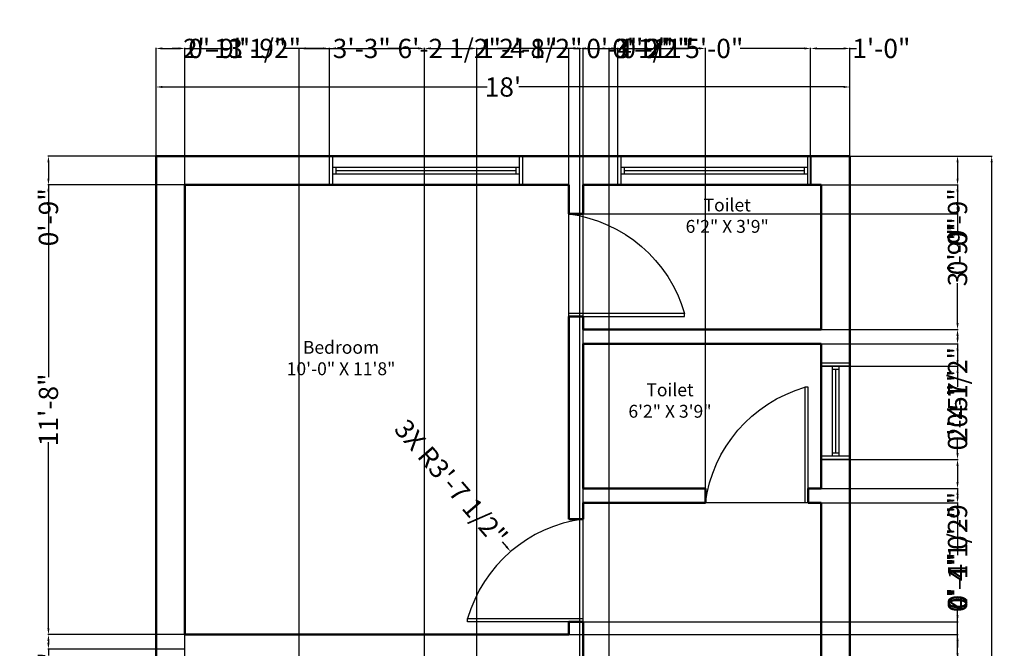
# Model space of a CAD drawing. Units: inches. Extents: x -34 to 296, y -84 to 618.
# Tile 3 of 3: x -11 to 296, y 423 to 618. Entities that reach past the tile are written whole.
import ezdxf

# ---------------------------------------------------------------- set-up
doc = ezdxf.new("R2010")
doc.units = ezdxf.units.IN
doc.header["$LTSCALE"] = 4
doc.header["$MEASUREMENT"] = 0
for name, color, linetype, lineweight in [('A-ANNO-DIMS', 2, 'Continuous', 18), ('A-AREA-IDEN', 3, 'Continuous', 18), ('A-DOOR', 4, 'Continuous', 25), ('A-GLAZ', 3, 'Continuous', 25), ('A-WALL', 7, 'Continuous', 50)]:
    doc.layers.add(name, color=color, linetype=linetype, lineweight=lineweight)
doc.styles.get("Standard").update_dxf_attribs({"font": 'arial.ttf'})
doc.dimstyles.get("Standard").update_dxf_attribs({"dimtxt": 6, "dimasz": 2, "dimexe": 0.18, "dimexo": 0.0625, "dimgap": 0.09, "dimtad": 0, "dimdec": 0, "dimzin": 0, "dimdsep": 46, "dimlunit": 4, "dimtxsty": 'Standard', "dimcen": 0.09, "dimadec": 0, "dimazin": 0, "dimtfac": 1, "dimtdec": 0, "dimtofl": 0, "dimtmove": 0, "dimatfit": 3, "dimfxl": 1, "dimtolj": 1, "dimtzin": 0, "dimarcsym": 0})

# ---------------------------------------------------------------- blocks, each defined once
blk = doc.blocks.new('*D1')
at = {"layer": 'A-ANNO-DIMS', "color": 0, "lineweight": -2, "transparency": 16777216}
for p, q in [((31.47, 576.1), (31.47, 597.71)), ((247.47, 576.1), (247.47, 597.71)), ((33.47, 597.53), (134.57, 597.53)), ((245.47, 597.53), (144.37, 597.53))]:
    blk.add_line(p, q, dxfattribs=at)
at = {"layer": 'A-ANNO-DIMS', "color": 0, "transparency": 16777216}
for points in [[(33.47, 597.86), (33.47, 597.2), (31.47, 597.53)], [(245.47, 597.86), (245.47, 597.2), (247.47, 597.53)]]:
    blk.add_solid(points, dxfattribs=at)
at = {"layer": 'Defpoints', "color": 0, "transparency": 16777216}
for p in [(247.47, 597.53), (31.47, 576.03), (247.47, 576.03)]:
    blk.add_point(p, dxfattribs=at)
at = {"layer": 'A-ANNO-DIMS', "color": 0, "transparency": 16777216, "insert": (139.47, 597.53), "char_height": 6, "attachment_point": 5}
blk.add_mtext("\\A1;18'", dxfattribs=at)
blk = doc.blocks.new('*D2')
at = {"layer": 'A-ANNO-DIMS', "color": 0, "lineweight": -2, "transparency": 16777216}
for p, q in [((247.53, 576.03), (291.77, 576.03)), ((291.59, 574.03), (291.59, 311.33)), ((291.59, 38.03), (291.59, 300.73)), ((247.53, 36.03), (291.77, 36.03))]:
    blk.add_line(p, q, dxfattribs=at)
at = {"layer": 'A-ANNO-DIMS', "color": 0, "transparency": 16777216}
for points in [[(291.26, 574.03), (291.92, 574.03), (291.59, 576.03)], [(291.26, 38.03), (291.92, 38.03), (291.59, 36.03)]]:
    blk.add_solid(points, dxfattribs=at)
at = {"layer": 'Defpoints', "color": 0, "transparency": 16777216}
for p in [(247.47, 576.03), (247.47, 36.03), (291.59, 36.03)]:
    blk.add_point(p, dxfattribs=at)
at = {"layer": 'A-ANNO-DIMS', "color": 0, "transparency": 16777216, "insert": (291.59, 306.03), "char_height": 6, "attachment_point": 5, "rotation": 90}
blk.add_mtext("\\A1;45'", dxfattribs=at)
blk = doc.blocks.new('DOOR')
for p, q in [((177.71, 683.29), (177.71, 692.29)), ((177.71, 692.29), (237.71, 692.29)), ((178.71, 683.29), (178.71, 692.29)), ((236.71, 692.29), (236.71, 683.29)), ((237.71, 692.29), (237.71, 683.29)), ((178.71, 688.79), (236.71, 688.79)), ((178.71, 686.79), (236.71, 686.79)), ((179.71, 686.79), (179.71, 688.79)), ((179.71, 687.79), (235.71, 687.79)), ((235.71, 688.79), (235.71, 686.79)), ((237.71, 683.29), (177.71, 683.29))]:
    blk.add_line(p, q)
blk = doc.blocks.new('DOOR-900')
for p, q in [((36, 0), (36, 32)), ((0, 0), (0, 1)), ((0, 1), (36, 1)), ((36, 0), (0, 0))]:
    blk.add_line(p, q)
blk.add_arc((41.68, -11), 43.37, 97.5204, 163.9438)
blk = doc.blocks.new('*D14')
at = {"layer": 'A-ANNO-DIMS', "color": 0, "lineweight": -2, "transparency": 16777216}
for p, q in [((31.47, 576.1), (31.47, 609.71)), ((33.47, 609.53), (38.47, 609.53)), ((40.47, 567.1), (40.47, 609.71)), ((40.47, 609.53), (42.47, 609.53))]:
    blk.add_line(p, q, dxfattribs=at)
at = {"layer": 'A-ANNO-DIMS', "color": 0, "transparency": 16777216}
for points in [[(33.47, 609.87), (33.47, 609.2), (31.47, 609.53)], [(38.47, 609.87), (38.47, 609.2), (40.47, 609.53)]]:
    blk.add_solid(points, dxfattribs=at)
at = {"layer": 'Defpoints', "color": 0, "transparency": 16777216}
for p in [(40.47, 609.53), (31.47, 576.03), (40.47, 567.03)]:
    blk.add_point(p, dxfattribs=at)
at = {"layer": 'A-ANNO-DIMS', "color": 0, "transparency": 16777216, "insert": (50.53, 609.53), "char_height": 6, "attachment_point": 5}
blk.add_mtext('\\A1;0\'-9"', dxfattribs=at)
blk = doc.blocks.new('*D15')
at = {"layer": 'A-ANNO-DIMS', "color": 0, "lineweight": -2, "transparency": 16777216}
for p, q in [((40.47, 567.1), (40.47, 609.71)), ((42.47, 609.53), (54.92, 609.53)), ((83.5, 609.53), (71.05, 609.53)), ((85.5, 567.1), (85.5, 609.71))]:
    blk.add_line(p, q, dxfattribs=at)
at = {"layer": 'A-ANNO-DIMS', "color": 0, "transparency": 16777216}
for points in [[(42.47, 609.87), (42.47, 609.2), (40.47, 609.53)], [(83.5, 609.87), (83.5, 609.2), (85.5, 609.53)]]:
    blk.add_solid(points, dxfattribs=at)
at = {"layer": 'Defpoints', "color": 0, "transparency": 16777216}
for p in [(85.5, 609.53), (40.47, 567.03), (85.5, 567.03)]:
    blk.add_point(p, dxfattribs=at)
at = {"layer": 'A-ANNO-DIMS', "color": 0, "transparency": 16777216, "insert": (62.99, 609.53), "char_height": 6, "attachment_point": 5}
blk.add_mtext('\\A1;3\'-9"', dxfattribs=at)
blk = doc.blocks.new('*D16')
at = {"layer": 'A-ANNO-DIMS', "color": 0, "lineweight": -2, "transparency": 16777216}
for p, q in [((85.5, 567.1), (85.5, 609.71)), ((87.5, 609.53), (107.66, 609.53)), ((157.97, 609.53), (137.81, 609.53)), ((159.97, 567.1), (159.97, 609.71))]:
    blk.add_line(p, q, dxfattribs=at)
at = {"layer": 'A-ANNO-DIMS', "color": 0, "transparency": 16777216}
for points in [[(87.5, 609.87), (87.5, 609.2), (85.5, 609.53)], [(157.97, 609.87), (157.97, 609.2), (159.97, 609.53)]]:
    blk.add_solid(points, dxfattribs=at)
at = {"layer": 'Defpoints', "color": 0, "transparency": 16777216}
for p in [(159.97, 609.53), (85.5, 567.03), (159.97, 567.03)]:
    blk.add_point(p, dxfattribs=at)
at = {"layer": 'A-ANNO-DIMS', "color": 0, "transparency": 16777216, "insert": (122.74, 609.53), "char_height": 6, "attachment_point": 5}
blk.add_mtext('\\A1;6\'-2 1/2"', dxfattribs=at)
blk = doc.blocks.new('*D17')
at = {"layer": 'A-ANNO-DIMS', "color": 0, "lineweight": -2, "transparency": 16777216}
for p, q in [((159.97, 567.1), (159.97, 609.71)), ((161.97, 609.53), (162.47, 609.53)), ((164.47, 567.1), (164.47, 609.71)), ((164.47, 609.53), (166.47, 609.53))]:
    blk.add_line(p, q, dxfattribs=at)
at = {"layer": 'A-ANNO-DIMS', "color": 0, "transparency": 16777216}
for points in [[(161.97, 609.87), (161.97, 609.2), (159.97, 609.53)], [(162.47, 609.87), (162.47, 609.2), (164.47, 609.53)]]:
    blk.add_solid(points, dxfattribs=at)
at = {"layer": 'Defpoints', "color": 0, "transparency": 16777216}
for p in [(164.47, 609.53), (159.97, 567.03), (164.47, 567.03)]:
    blk.add_point(p, dxfattribs=at)
at = {"layer": 'A-ANNO-DIMS', "color": 0, "transparency": 16777216, "insert": (181.52, 609.53), "char_height": 6, "attachment_point": 5}
blk.add_mtext('\\A1;0\'-4 1/2"', dxfattribs=at)
blk = doc.blocks.new('*D18')
at = {"layer": 'A-ANNO-DIMS', "color": 0, "lineweight": -2, "transparency": 16777216}
for p, q in [((164.47, 567.1), (164.47, 609.71)), ((166.47, 609.53), (173.24, 609.53)), ((175.24, 567.1), (175.24, 609.71)), ((175.24, 609.53), (177.24, 609.53))]:
    blk.add_line(p, q, dxfattribs=at)
at = {"layer": 'A-ANNO-DIMS', "color": 0, "transparency": 16777216}
for points in [[(166.47, 609.87), (166.47, 609.2), (164.47, 609.53)], [(173.24, 609.87), (173.24, 609.2), (175.24, 609.53)]]:
    blk.add_solid(points, dxfattribs=at)
at = {"layer": 'Defpoints', "color": 0, "transparency": 16777216}
for p in [(175.24, 609.53), (164.47, 567.03), (175.24, 567.03)]:
    blk.add_point(p, dxfattribs=at)
at = {"layer": 'A-ANNO-DIMS', "color": 0, "transparency": 16777216, "insert": (187.64, 609.53), "char_height": 6, "attachment_point": 5}
blk.add_mtext('\\A1;0\'-11"', dxfattribs=at)
blk = doc.blocks.new('*D19')
at = {"layer": 'A-ANNO-DIMS', "color": 0, "lineweight": -2, "transparency": 16777216}
for p, q in [((175.24, 567.1), (175.24, 609.71)), ((177.24, 609.53), (197.18, 609.53)), ((233.24, 609.53), (213.31, 609.53)), ((235.24, 567.1), (235.24, 609.71))]:
    blk.add_line(p, q, dxfattribs=at)
at = {"layer": 'A-ANNO-DIMS', "color": 0, "transparency": 16777216}
for points in [[(177.24, 609.87), (177.24, 609.2), (175.24, 609.53)], [(233.24, 609.87), (233.24, 609.2), (235.24, 609.53)]]:
    blk.add_solid(points, dxfattribs=at)
at = {"layer": 'Defpoints', "color": 0, "transparency": 16777216}
for p in [(235.24, 609.53), (175.24, 567.03), (235.24, 567.03)]:
    blk.add_point(p, dxfattribs=at)
at = {"layer": 'A-ANNO-DIMS', "color": 0, "transparency": 16777216, "insert": (205.24, 609.53), "char_height": 6, "attachment_point": 5}
blk.add_mtext('\\A1;5\'-0"', dxfattribs=at)
blk = doc.blocks.new('*D20')
at = {"layer": 'A-ANNO-DIMS', "color": 0, "lineweight": -2, "transparency": 16777216}
for p, q in [((235.24, 567.1), (235.24, 609.71)), ((237.24, 609.53), (245.47, 609.53)), ((247.47, 576.1), (247.47, 609.71)), ((247.47, 609.53), (249.47, 609.53))]:
    blk.add_line(p, q, dxfattribs=at)
at = {"layer": 'A-ANNO-DIMS', "color": 0, "transparency": 16777216}
for points in [[(237.24, 609.87), (237.24, 609.2), (235.24, 609.53)], [(245.47, 609.87), (245.47, 609.2), (247.47, 609.53)]]:
    blk.add_solid(points, dxfattribs=at)
at = {"layer": 'Defpoints', "color": 0, "transparency": 16777216}
for p in [(247.47, 609.53), (247.47, 576.03), (235.24, 567.03)]:
    blk.add_point(p, dxfattribs=at)
at = {"layer": 'A-ANNO-DIMS', "color": 0, "transparency": 16777216, "insert": (257.25, 609.53), "char_height": 6, "attachment_point": 5}
blk.add_mtext('\\A1;1\'-0"', dxfattribs=at)
blk = doc.blocks.new('*D21')
at = {"layer": 'A-ANNO-DIMS', "color": 0, "lineweight": -2, "transparency": 16777216}
for p, q in [((31.4, 576.03), (-2.21, 576.03)), ((-2.03, 574.03), (-2.03, 569.03)), ((40.4, 567.03), (-2.21, 567.03)), ((-2.03, 567.03), (-2.03, 565.03))]:
    blk.add_line(p, q, dxfattribs=at)
at = {"layer": 'A-ANNO-DIMS', "color": 0, "transparency": 16777216}
for points in [[(-2.37, 574.03), (-1.7, 574.03), (-2.03, 576.03)], [(-2.37, 569.03), (-1.7, 569.03), (-2.03, 567.03)]]:
    blk.add_solid(points, dxfattribs=at)
at = {"layer": 'Defpoints', "color": 0, "transparency": 16777216}
for p in [(31.47, 576.03), (-2.03, 567.03), (40.47, 567.03)]:
    blk.add_point(p, dxfattribs=at)
at = {"layer": 'A-ANNO-DIMS', "color": 0, "transparency": 16777216, "insert": (-2.03, 556.97), "char_height": 6, "attachment_point": 5, "rotation": 90}
blk.add_mtext('\\A1;0\'-9"', dxfattribs=at)
blk = doc.blocks.new('*D22')
at = {"layer": 'A-ANNO-DIMS', "color": 0, "lineweight": -2, "transparency": 16777216}
for p, q in [((40.4, 567.03), (-2.21, 567.03)), ((-2.03, 565.03), (-2.03, 507.15)), ((-2.03, 429.03), (-2.03, 486.92)), ((40.4, 427.03), (-2.21, 427.03))]:
    blk.add_line(p, q, dxfattribs=at)
at = {"layer": 'A-ANNO-DIMS', "color": 0, "transparency": 16777216}
for points in [[(-2.37, 565.03), (-1.7, 565.03), (-2.03, 567.03)], [(-2.37, 429.03), (-1.7, 429.03), (-2.03, 427.03)]]:
    blk.add_solid(points, dxfattribs=at)
at = {"layer": 'Defpoints', "color": 0, "transparency": 16777216}
for p in [(40.47, 567.03), (-2.03, 427.03), (40.47, 427.03)]:
    blk.add_point(p, dxfattribs=at)
at = {"layer": 'A-ANNO-DIMS', "color": 0, "transparency": 16777216, "insert": (-2.03, 497.03), "char_height": 6, "attachment_point": 5, "rotation": 90}
blk.add_mtext('\\A1;11\'-8"', dxfattribs=at)
blk = doc.blocks.new('*D23')
at = {"layer": 'A-ANNO-DIMS', "color": 0, "lineweight": -2, "transparency": 16777216}
for p, q in [((40.4, 427.03), (-2.21, 427.03)), ((-2.03, 425.03), (-2.03, 424.53)), ((40.4, 422.53), (-2.21, 422.53)), ((-2.03, 422.53), (-2.03, 420.53))]:
    blk.add_line(p, q, dxfattribs=at)
at = {"layer": 'A-ANNO-DIMS', "color": 0, "transparency": 16777216}
for points in [[(-2.37, 425.03), (-1.7, 425.03), (-2.03, 427.03)], [(-2.37, 424.53), (-1.7, 424.53), (-2.03, 422.53)]]:
    blk.add_solid(points, dxfattribs=at)
at = {"layer": 'Defpoints', "color": 0, "transparency": 16777216}
for p in [(40.47, 427.03), (-2.03, 422.53), (40.47, 422.53)]:
    blk.add_point(p, dxfattribs=at)
at = {"layer": 'A-ANNO-DIMS', "color": 0, "transparency": 16777216, "insert": (-2.03, 405.48), "char_height": 6, "attachment_point": 5, "rotation": 90}
blk.add_mtext('\\A1;0\'-4 1/2"', dxfattribs=at)
blk = doc.blocks.new('*D29')
at = {"layer": 'A-ANNO-DIMS', "color": 0, "lineweight": -2, "transparency": 16777216}
for p, q in [((247.53, 576.03), (281.15, 576.03)), ((280.97, 574.03), (280.97, 569.03)), ((238.53, 567.03), (281.15, 567.03)), ((280.97, 567.03), (280.97, 565.03))]:
    blk.add_line(p, q, dxfattribs=at)
at = {"layer": 'A-ANNO-DIMS', "color": 0, "transparency": 16777216}
for points in [[(280.63, 574.03), (281.3, 574.03), (280.97, 576.03)], [(280.63, 569.03), (281.3, 569.03), (280.97, 567.03)]]:
    blk.add_solid(points, dxfattribs=at)
at = {"layer": 'Defpoints', "color": 0, "transparency": 16777216}
for p in [(247.47, 576.03), (238.47, 567.03), (280.97, 567.03)]:
    blk.add_point(p, dxfattribs=at)
at = {"layer": 'A-ANNO-DIMS', "color": 0, "transparency": 16777216, "insert": (280.97, 556.97), "char_height": 6, "attachment_point": 5, "rotation": 90}
blk.add_mtext('\\A1;0\'-9"', dxfattribs=at)
blk = doc.blocks.new('*D30')
at = {"layer": 'A-ANNO-DIMS', "color": 0, "lineweight": -2, "transparency": 16777216}
for p, q in [((238.53, 567.03), (281.15, 567.03)), ((280.97, 565.03), (280.97, 552.6)), ((280.97, 524.03), (280.97, 536.47)), ((238.53, 522.03), (281.15, 522.03))]:
    blk.add_line(p, q, dxfattribs=at)
at = {"layer": 'A-ANNO-DIMS', "color": 0, "transparency": 16777216}
for points in [[(280.63, 565.03), (281.3, 565.03), (280.97, 567.03)], [(280.63, 524.03), (281.3, 524.03), (280.97, 522.03)]]:
    blk.add_solid(points, dxfattribs=at)
at = {"layer": 'Defpoints', "color": 0, "transparency": 16777216}
for p in [(238.47, 567.03), (238.47, 522.03), (280.97, 522.03)]:
    blk.add_point(p, dxfattribs=at)
at = {"layer": 'A-ANNO-DIMS', "color": 0, "transparency": 16777216, "insert": (280.97, 544.53), "char_height": 6, "attachment_point": 5, "rotation": 90}
blk.add_mtext('\\A1;3\'-9"', dxfattribs=at)
blk = doc.blocks.new('*D31')
at = {"layer": 'A-ANNO-DIMS', "color": 0, "lineweight": -2, "transparency": 16777216}
for p, q in [((238.53, 522.03), (281.15, 522.03)), ((280.97, 520.03), (280.97, 519.53)), ((238.53, 517.53), (281.15, 517.53)), ((280.97, 517.53), (280.97, 515.53))]:
    blk.add_line(p, q, dxfattribs=at)
at = {"layer": 'A-ANNO-DIMS', "color": 0, "transparency": 16777216}
for points in [[(280.63, 520.03), (281.3, 520.03), (280.97, 522.03)], [(280.63, 519.53), (281.3, 519.53), (280.97, 517.53)]]:
    blk.add_solid(points, dxfattribs=at)
at = {"layer": 'Defpoints', "color": 0, "transparency": 16777216}
for p in [(238.47, 522.03), (238.47, 517.53), (280.97, 517.53)]:
    blk.add_point(p, dxfattribs=at)
at = {"layer": 'A-ANNO-DIMS', "color": 0, "transparency": 16777216, "insert": (280.97, 500.48), "char_height": 6, "attachment_point": 5, "rotation": 90}
blk.add_mtext('\\A1;0\'-4 1/2"', dxfattribs=at)
blk = doc.blocks.new('*D32')
at = {"layer": 'A-ANNO-DIMS', "color": 0, "lineweight": -2, "transparency": 16777216}
for p, q in [((238.53, 517.53), (281.15, 517.53)), ((280.97, 515.53), (280.97, 512.57)), ((238.53, 510.57), (281.15, 510.57)), ((280.97, 510.57), (280.97, 508.57))]:
    blk.add_line(p, q, dxfattribs=at)
at = {"layer": 'A-ANNO-DIMS', "color": 0, "transparency": 16777216}
for points in [[(280.63, 515.53), (281.3, 515.53), (280.97, 517.53)], [(280.63, 512.57), (281.3, 512.57), (280.97, 510.57)]]:
    blk.add_solid(points, dxfattribs=at)
at = {"layer": 'Defpoints', "color": 0, "transparency": 16777216}
for p in [(238.47, 517.53), (238.47, 510.57), (280.97, 510.57)]:
    blk.add_point(p, dxfattribs=at)
at = {"layer": 'A-ANNO-DIMS', "color": 0, "transparency": 16777216, "insert": (280.97, 500.5), "char_height": 6, "attachment_point": 5, "rotation": 90}
blk.add_mtext('\\A1;0\'-7"', dxfattribs=at)
blk = doc.blocks.new('*D33')
at = {"layer": 'A-ANNO-DIMS', "color": 0, "lineweight": -2, "transparency": 16777216}
for p, q in [((238.53, 510.57), (281.15, 510.57)), ((280.97, 508.57), (280.97, 504.18)), ((280.97, 483.57), (280.97, 487.95)), ((238.53, 481.57), (281.15, 481.57))]:
    blk.add_line(p, q, dxfattribs=at)
at = {"layer": 'A-ANNO-DIMS', "color": 0, "transparency": 16777216}
for points in [[(280.63, 508.57), (281.3, 508.57), (280.97, 510.57)], [(280.63, 483.57), (281.3, 483.57), (280.97, 481.57)]]:
    blk.add_solid(points, dxfattribs=at)
at = {"layer": 'Defpoints', "color": 0, "transparency": 16777216}
for p in [(238.47, 510.57), (238.47, 481.57), (280.97, 481.57)]:
    blk.add_point(p, dxfattribs=at)
at = {"layer": 'A-ANNO-DIMS', "color": 0, "transparency": 16777216, "insert": (280.97, 496.07), "char_height": 6, "attachment_point": 5, "rotation": 90}
blk.add_mtext('\\A1;2\'-5"', dxfattribs=at)
blk = doc.blocks.new('*D34')
at = {"layer": 'A-ANNO-DIMS', "color": 0, "lineweight": -2, "transparency": 16777216}
for p, q in [((238.53, 481.57), (281.15, 481.57)), ((280.97, 479.57), (280.97, 474.53)), ((238.53, 472.53), (281.15, 472.53)), ((280.97, 472.53), (280.97, 470.53))]:
    blk.add_line(p, q, dxfattribs=at)
at = {"layer": 'A-ANNO-DIMS', "color": 0, "transparency": 16777216}
for points in [[(280.63, 479.57), (281.3, 479.57), (280.97, 481.57)], [(280.63, 474.53), (281.3, 474.53), (280.97, 472.53)]]:
    blk.add_solid(points, dxfattribs=at)
at = {"layer": 'Defpoints', "color": 0, "transparency": 16777216}
for p in [(238.47, 481.57), (238.47, 472.53), (280.97, 472.53)]:
    blk.add_point(p, dxfattribs=at)
at = {"layer": 'A-ANNO-DIMS', "color": 0, "transparency": 16777216, "insert": (280.97, 462.47), "char_height": 6, "attachment_point": 5, "rotation": 90}
blk.add_mtext('\\A1;0\'-9"', dxfattribs=at)
blk = doc.blocks.new('*D35')
at = {"layer": 'A-ANNO-DIMS', "color": 0, "lineweight": -2, "transparency": 16777216}
for p, q in [((238.53, 472.53), (281.15, 472.53)), ((280.97, 470.53), (280.97, 470.03)), ((238.53, 468.03), (281.15, 468.03)), ((280.97, 468.03), (280.97, 466.03))]:
    blk.add_line(p, q, dxfattribs=at)
at = {"layer": 'A-ANNO-DIMS', "color": 0, "transparency": 16777216}
for points in [[(280.63, 470.53), (281.3, 470.53), (280.97, 472.53)], [(280.63, 470.03), (281.3, 470.03), (280.97, 468.03)]]:
    blk.add_solid(points, dxfattribs=at)
at = {"layer": 'Defpoints', "color": 0, "transparency": 16777216}
for p in [(238.47, 472.53), (238.47, 468.03), (280.97, 468.03)]:
    blk.add_point(p, dxfattribs=at)
at = {"layer": 'A-ANNO-DIMS', "color": 0, "transparency": 16777216, "insert": (280.97, 450.98), "char_height": 6, "attachment_point": 5, "rotation": 90}
blk.add_mtext('\\A1;0\'-4 1/2"', dxfattribs=at)
blk = doc.blocks.new('*D36')
at = {"layer": 'A-ANNO-DIMS', "color": 0, "lineweight": -2, "transparency": 16777216}
for p, q in [((238.53, 468.03), (281.15, 468.03)), ((280.97, 466.03), (280.97, 451.82)), ((280.97, 421.24), (280.97, 435.45)), ((238.53, 419.24), (281.15, 419.24))]:
    blk.add_line(p, q, dxfattribs=at)
at = {"layer": 'A-ANNO-DIMS', "color": 0, "transparency": 16777216}
for points in [[(280.63, 466.03), (281.3, 466.03), (280.97, 468.03)], [(280.63, 421.24), (281.3, 421.24), (280.97, 419.24)]]:
    blk.add_solid(points, dxfattribs=at)
at = {"layer": 'Defpoints', "color": 0, "transparency": 16777216}
for p in [(238.47, 468.03), (238.47, 419.24), (280.97, 419.24)]:
    blk.add_point(p, dxfattribs=at)
at = {"layer": 'A-ANNO-DIMS', "color": 0, "transparency": 16777216, "insert": (280.97, 443.63), "char_height": 6, "attachment_point": 5, "rotation": 90}
blk.add_mtext('\\A1;4\'-1"', dxfattribs=at)
blk = doc.blocks.new('*D41')
at = {"layer": 'A-ANNO-DIMS', "color": 0, "lineweight": -2, "transparency": 16777216}
for p, q in [((164.53, 567.03), (281.15, 567.03)), ((280.97, 565.03), (280.97, 560.03)), ((164.53, 558.03), (281.15, 558.03)), ((280.97, 558.03), (280.97, 556.03))]:
    blk.add_line(p, q, dxfattribs=at)
at = {"layer": 'A-ANNO-DIMS', "color": 0, "transparency": 16777216}
for points in [[(280.63, 565.03), (281.3, 565.03), (280.97, 567.03)], [(280.63, 560.03), (281.3, 560.03), (280.97, 558.03)]]:
    blk.add_solid(points, dxfattribs=at)
at = {"layer": 'Defpoints', "color": 0, "transparency": 16777216}
for p in [(164.47, 567.03), (164.47, 558.03), (280.97, 558.03)]:
    blk.add_point(p, dxfattribs=at)
at = {"layer": 'A-ANNO-DIMS', "color": 0, "transparency": 16777216, "insert": (280.97, 547.97), "char_height": 6, "attachment_point": 5, "rotation": 90}
blk.add_mtext('\\A1;0\'-9"', dxfattribs=at)
blk = doc.blocks.new('*D42')
at = {"layer": 'A-ANNO-DIMS', "color": 0, "lineweight": -2, "transparency": 16777216}
for p, q in [((280.97, 433.03), (280.97, 435.03)), ((160.03, 431.03), (281.15, 431.03)), ((160.03, 427.03), (281.15, 427.03)), ((280.97, 425.03), (280.97, 423.03))]:
    blk.add_line(p, q, dxfattribs=at)
at = {"layer": 'A-ANNO-DIMS', "color": 0, "transparency": 16777216}
for points in [[(280.63, 433.03), (281.3, 433.03), (280.97, 431.03)], [(280.63, 425.03), (281.3, 425.03), (280.97, 427.03)]]:
    blk.add_solid(points, dxfattribs=at)
at = {"layer": 'Defpoints', "color": 0, "transparency": 16777216}
for p in [(159.97, 431.03), (280.97, 431.03), (159.97, 427.03)]:
    blk.add_point(p, dxfattribs=at)
at = {"layer": 'A-ANNO-DIMS', "color": 0, "transparency": 16777216, "insert": (280.97, 443.1), "char_height": 6, "attachment_point": 5, "rotation": 90}
blk.add_mtext('\\A1;0\'-4"', dxfattribs=at)
blk = doc.blocks.new('*D43')
at = {"layer": 'A-ANNO-DIMS', "color": 0, "lineweight": -2, "transparency": 16777216}
for p, q in [((164.47, 468.1), (164.47, 609.71)), ((166.47, 609.53), (175.4, 609.53)), ((200.47, 609.53), (191.53, 609.53)), ((202.47, 468.1), (202.47, 609.71))]:
    blk.add_line(p, q, dxfattribs=at)
at = {"layer": 'A-ANNO-DIMS', "color": 0, "transparency": 16777216}
for points in [[(166.47, 609.87), (166.47, 609.2), (164.47, 609.53)], [(200.47, 609.87), (200.47, 609.2), (202.47, 609.53)]]:
    blk.add_solid(points, dxfattribs=at)
at = {"layer": 'Defpoints', "color": 0, "transparency": 16777216}
for p in [(202.47, 609.53), (164.47, 468.03), (202.47, 468.03)]:
    blk.add_point(p, dxfattribs=at)
at = {"layer": 'A-ANNO-DIMS', "color": 0, "transparency": 16777216, "insert": (183.47, 609.53), "char_height": 6, "attachment_point": 5}
blk.add_mtext('\\A1;3\'-2"', dxfattribs=at)
blk = doc.blocks.new('*D51')
at = {"layer": 'A-ANNO-DIMS', "color": 0, "lineweight": -2, "transparency": 16777216}
for p, q in [((38.47, 609.53), (36.47, 609.53)), ((40.47, 129.6), (40.47, 609.71)), ((76.01, 129.6), (76.01, 609.71)), ((78.01, 609.53), (80.01, 609.53))]:
    blk.add_line(p, q, dxfattribs=at)
at = {"layer": 'A-ANNO-DIMS', "color": 0, "transparency": 16777216}
for points in [[(38.47, 609.87), (38.47, 609.2), (40.47, 609.53)], [(78.01, 609.87), (78.01, 609.2), (76.01, 609.53)]]:
    blk.add_solid(points, dxfattribs=at)
at = {"layer": 'Defpoints', "color": 0, "transparency": 16777216}
for p in [(76.01, 609.53), (40.47, 129.53), (76.01, 129.53)]:
    blk.add_point(p, dxfattribs=at)
at = {"layer": 'A-ANNO-DIMS', "color": 0, "transparency": 16777216, "insert": (58.24, 609.53), "char_height": 6, "attachment_point": 5}
blk.add_mtext('\\A1;2\'-11 1/2"', dxfattribs=at)
blk = doc.blocks.new('*D52')
at = {"layer": 'A-ANNO-DIMS', "color": 0, "lineweight": -2, "transparency": 16777216}
for p, q in [((76.01, 129.6), (76.01, 609.71)), ((78.01, 609.53), (87.45, 609.53)), ((113.01, 609.53), (103.57, 609.53)), ((115.01, 129.6), (115.01, 609.71))]:
    blk.add_line(p, q, dxfattribs=at)
at = {"layer": 'A-ANNO-DIMS', "color": 0, "transparency": 16777216}
for points in [[(78.01, 609.87), (78.01, 609.2), (76.01, 609.53)], [(113.01, 609.87), (113.01, 609.2), (115.01, 609.53)]]:
    blk.add_solid(points, dxfattribs=at)
at = {"layer": 'Defpoints', "color": 0, "transparency": 16777216}
for p in [(115.01, 609.53), (76.01, 129.53), (115.01, 129.53)]:
    blk.add_point(p, dxfattribs=at)
at = {"layer": 'A-ANNO-DIMS', "color": 0, "transparency": 16777216, "insert": (95.51, 609.53), "char_height": 6, "attachment_point": 5}
blk.add_mtext('\\A1;3\'-3"', dxfattribs=at)
blk = doc.blocks.new('*D53')
at = {"layer": 'A-ANNO-DIMS', "color": 0, "lineweight": -2, "transparency": 16777216}
for p, q in [((115.01, 129.6), (115.01, 609.71)), ((117.01, 609.53), (129.36, 609.53)), ((131.36, 129.6), (131.36, 609.71)), ((131.36, 609.53), (133.36, 609.53))]:
    blk.add_line(p, q, dxfattribs=at)
at = {"layer": 'A-ANNO-DIMS', "color": 0, "transparency": 16777216}
for points in [[(117.01, 609.87), (117.01, 609.2), (115.01, 609.53)], [(129.36, 609.87), (129.36, 609.2), (131.36, 609.53)]]:
    blk.add_solid(points, dxfattribs=at)
at = {"layer": 'Defpoints', "color": 0, "transparency": 16777216}
for p in [(131.36, 609.53), (115.01, 129.53), (131.36, 129.53)]:
    blk.add_point(p, dxfattribs=at)
at = {"layer": 'A-ANNO-DIMS', "color": 0, "transparency": 16777216, "insert": (148.13, 609.53), "char_height": 6, "attachment_point": 5}
blk.add_mtext('\\A1;1\'-4 1/2"', dxfattribs=at)
blk = doc.blocks.new('*D54')
at = {"layer": 'A-ANNO-DIMS', "color": 0, "lineweight": -2, "transparency": 16777216}
for p, q in [((131.36, 129.6), (131.36, 609.71)), ((133.36, 609.53), (139.24, 609.53)), ((161.36, 609.53), (155.48, 609.53)), ((163.36, 129.6), (163.36, 609.71))]:
    blk.add_line(p, q, dxfattribs=at)
at = {"layer": 'A-ANNO-DIMS', "color": 0, "transparency": 16777216}
for points in [[(133.36, 609.87), (133.36, 609.2), (131.36, 609.53)], [(161.36, 609.87), (161.36, 609.2), (163.36, 609.53)]]:
    blk.add_solid(points, dxfattribs=at)
at = {"layer": 'Defpoints', "color": 0, "transparency": 16777216}
for p in [(163.36, 609.53), (131.36, 129.53), (163.36, 129.53)]:
    blk.add_point(p, dxfattribs=at)
at = {"layer": 'A-ANNO-DIMS', "color": 0, "transparency": 16777216, "insert": (147.36, 609.53), "char_height": 6, "attachment_point": 5}
blk.add_mtext('\\A1;2\'-8"', dxfattribs=at)
blk = doc.blocks.new('*D55')
at = {"layer": 'A-ANNO-DIMS', "color": 0, "lineweight": -2, "transparency": 16777216}
for p, q in [((163.36, 129.6), (163.36, 609.71)), ((165.36, 609.53), (170.47, 609.53)), ((172.47, 129.6), (172.47, 609.71)), ((172.47, 609.53), (174.47, 609.53))]:
    blk.add_line(p, q, dxfattribs=at)
at = {"layer": 'A-ANNO-DIMS', "color": 0, "transparency": 16777216}
for points in [[(165.36, 609.87), (165.36, 609.2), (163.36, 609.53)], [(170.47, 609.87), (170.47, 609.2), (172.47, 609.53)]]:
    blk.add_solid(points, dxfattribs=at)
at = {"layer": 'Defpoints', "color": 0, "transparency": 16777216}
for p in [(172.47, 609.53), (163.36, 129.53), (172.47, 129.53)]:
    blk.add_point(p, dxfattribs=at)
at = {"layer": 'A-ANNO-DIMS', "color": 0, "transparency": 16777216, "insert": (182.53, 609.53), "char_height": 6, "attachment_point": 5}
blk.add_mtext('\\A1;0\'-9"', dxfattribs=at)
blk = doc.blocks.new('*D59')
at = {"layer": 'A-ANNO-DIMS', "color": 0, "lineweight": -2, "transparency": 16777216}
for p, q in [((139.23, 455.93), (140.54, 454.42)), ((170.05, 420.04), (170.23, 420.04)), ((170.14, 419.95), (170.14, 420.13))]:
    blk.add_line(p, q, dxfattribs=at)
at = {"layer": 'A-ANNO-DIMS', "color": 0, "transparency": 16777216}
blk.add_solid([(140.79, 454.63), (140.29, 454.2), (141.84, 452.9)], dxfattribs=at)
at = {"layer": 'Defpoints', "color": 0, "transparency": 16777216}
for p in [(141.84, 452.9), (170.14, 420.04)]:
    blk.add_point(p, dxfattribs=at)
at = {"layer": 'A-ANNO-DIMS', "color": 0, "transparency": 16777216, "insert": (123.33, 474.4), "char_height": 6, "attachment_point": 5, "rotation": 310.7319}
blk.add_mtext('\\A1;3X R3\'-7 1/2"', dxfattribs=at)

msp = doc.modelspace()

# ---------------------------------------------------------------- linework, layer by layer
at = {"layer": 'A-GLAZ'}
for p, q in [((247.47, 511.57), (238.47, 511.57)), ((247.47, 510.57), (238.47, 510.57)), ((241.97, 510.57), (241.97, 482.57)), ((243.97, 509.57), (241.97, 509.57)), ((242.97, 509.57), (242.97, 483.57)), ((243.97, 510.57), (243.97, 482.57)), ((247.47, 482.57), (238.47, 482.57)), ((247.47, 481.57), (238.47, 481.57)), ((243.97, 483.57), (241.97, 483.57))]:
    msp.add_line(p, q, dxfattribs=at)
at = {"layer": 'A-WALL'}
for p, q in [((31.47, 576.03), (247.47, 576.03)), ((31.47, 36.03), (31.47, 576.03)), ((247.47, 576.03), (247.47, 36.03)), ((40.47, 567.03), (159.97, 567.03)), ((40.47, 427.03), (40.47, 567.03)), ((159.97, 567.03), (159.97, 558.03)), ((164.47, 567.03), (164.47, 558.03)), ((164.47, 567.03), (238.47, 567.03)), ((238.47, 567.03), (238.47, 522.03)), ((159.97, 558.03), (164.47, 558.03)), ((159.97, 526.03), (164.47, 526.03)), ((159.97, 526.03), (159.97, 463.03)), ((164.47, 526.03), (164.47, 522.03)), ((164.47, 522.03), (238.47, 522.03)), ((164.47, 517.53), (238.47, 517.53)), ((164.47, 517.53), (164.47, 472.53)), ((238.47, 517.53), (238.47, 472.53)), ((164.47, 472.53), (202.47, 472.53)), ((202.47, 472.53), (202.47, 468.03)), ((234.47, 472.53), (234.47, 468.03)), ((234.47, 472.53), (238.47, 472.53)), ((164.47, 468.03), (202.47, 468.03)), ((164.47, 468.03), (164.47, 463.03)), ((234.47, 468.03), (238.47, 468.03)), ((238.47, 468.03), (238.47, 45.03)), ((159.97, 463.03), (164.47, 463.03)), ((159.97, 431.03), (164.47, 431.03)), ((159.97, 431.03), (159.97, 427.03)), ((164.47, 431.03), (164.47, 318.53)), ((40.47, 427.03), (159.97, 427.03))]:
    msp.add_line(p, q, dxfattribs=at)

# ---------------------------------------------------------------- block references
at = {"layer": 'A-DOOR', "extrusion": (0, 0, -1), "zscale": -1}
msp.add_blockref('DOOR-900', (-195.97, 526.03), dxfattribs=at)
at = {"layer": 'A-DOOR', "extrusion": (0, 0, -1), "zscale": -1, "rotation": 270}
msp.add_blockref('DOOR-900', (-234.47, 504.03), dxfattribs=at)
at = {"layer": 'A-DOOR'}
msp.add_blockref('DOOR-900', (128.47, 431.03), dxfattribs=at)
at = {"layer": 'A-GLAZ'}
for p in [(-92.2, -116.26), (-2.46, -116.26)]:
    msp.add_blockref('DOOR', p, dxfattribs=at)

# ---------------------------------------------------------------- texts
at = {"layer": 'A-AREA-IDEN', "char_height": 4, "attachment_point": 1}
for s, width, insert in [('\\pxqc;Toilet\\P6\'2" X 3\'9"', 51.6816, (183.42, 562.8)), ('\\pxqc;Bedroom\\P10\'-0" X 11\'8"', 62.1792, (57.97, 518.48)), ('\\pxqc;Toilet\\P6\'2" X 3\'9"', 51.6816, (165.61, 505.24))]:
    msp.add_mtext_dynamic_manual_height_columns(s, width=width, gutter_width=20, heights=[0], dxfattribs=dict(at, insert=insert))

# ---------------------------------------------------------------- dimensions: what is measured, and where the dimension line sits
at = {"layer": 'A-ANNO-DIMS'}
for base, p1, p2, override, picture, middle in [((76.01, 609.53), (40.47, 129.53), (76.01, 129.53), {"dimdec": 1, "dimlfac": 1, "dimrnd": 0, "dimzin": 1, "dimdsep": 46, "dimlunit": 4, "dimfrac": 2}, '*D51', (58.24, 609.53)), ((159.97, 609.53), (85.5, 567.03), (159.97, 567.03), {"dimdec": 1, "dimlfac": 1, "dimrnd": 0, "dimzin": 1, "dimdsep": 46, "dimlunit": 4, "dimfrac": 2}, '*D16', (122.74, 609.53)), ((131.3602, 609.5325), (115.0111, 129.5325), (131.3602, 129.5325), {"dimdec": 1, "dimlfac": 1, "dimrnd": 0, "dimzin": 1, "dimdsep": 46, "dimlunit": 4, "dimfrac": 2}, '*D53', (148.133, 609.5325)), ((164.47, 609.53), (159.97, 567.03), (164.47, 567.03), {"dimdec": 1, "dimlfac": 1, "dimrnd": 0, "dimzin": 1, "dimdsep": 46, "dimlunit": 4, "dimfrac": 2}, '*D17', (181.52, 609.53)), ((40.47, 609.53), (31.47, 576.03), (40.47, 567.03), {"dimdec": 1, "dimlfac": 1, "dimrnd": 0, "dimzin": 1, "dimdsep": 46, "dimlunit": 4, "dimfrac": 2}, '*D14', (50.53, 609.53)), ((85.5, 609.53), (40.47, 567.03), (85.5, 567.03), {"dimdec": 1, "dimlfac": 1, "dimrnd": 0, "dimzin": 1, "dimdsep": 46, "dimlunit": 4, "dimfrac": 2}, '*D15', (62.99, 609.53)), ((115.01, 609.53), (76.01, 129.53), (115.01, 129.53), {"dimdec": 1, "dimlfac": 1, "dimrnd": 0, "dimzin": 1, "dimdsep": 46, "dimlunit": 4, "dimfrac": 2}, '*D52', (95.51, 609.53)), ((163.36, 609.53), (131.36, 129.53), (163.36, 129.53), {"dimdec": 1, "dimlfac": 1, "dimrnd": 0, "dimzin": 1, "dimdsep": 46, "dimlunit": 4, "dimfrac": 2}, '*D54', (147.36, 609.53)), ((172.47, 609.53), (163.36, 129.53), (172.47, 129.53), {"dimdec": 1, "dimlfac": 1, "dimrnd": 0, "dimzin": 1, "dimdsep": 46, "dimlunit": 4, "dimfrac": 2}, '*D55', (182.53, 609.53)), ((175.24, 609.53), (164.47, 567.03), (175.24, 567.03), {"dimdec": 1, "dimlfac": 1, "dimrnd": 0, "dimzin": 1, "dimdsep": 46, "dimlunit": 4, "dimfrac": 2}, '*D18', (187.64, 609.53)), ((202.47, 609.53), (164.47, 468.03), (202.47, 468.03), {"dimdec": 1, "dimlfac": 1, "dimrnd": 0, "dimzin": 1, "dimdsep": 46, "dimlunit": 4, "dimfrac": 2}, '*D43', (183.47, 609.53)), ((235.24, 609.53), (175.24, 567.03), (235.24, 567.03), {"dimdec": 1, "dimlfac": 1, "dimrnd": 0, "dimzin": 1, "dimdsep": 46, "dimlunit": 4, "dimfrac": 2}, '*D19', (205.24, 609.53)), ((247.47, 609.53), (235.24, 567.03), (247.47, 576.03), {"dimdec": 1, "dimlfac": 1, "dimrnd": 0, "dimzin": 1, "dimdsep": 46, "dimlunit": 4, "dimfrac": 2}, '*D20', (257.25, 609.53)), ((247.47, 597.53), (31.47, 576.03), (247.47, 576.03), {"dimclrd": 0, "dimclre": 0, "dimclrt": 0}, '*D1', (139.47, 597.53))]:
    dim = msp.add_linear_dim(base=base, p1=p1, p2=p2, dimstyle='Standard', override=override, dxfattribs=at)
    dim.commit()
    dim.dimension.update_dxf_attribs({"geometry": picture, "text_midpoint": middle})
for base, p1, p2, override, picture, middle in [((-2.03, 567.03), (31.47, 576.03), (40.47, 567.03), {"dimdec": 1, "dimlfac": 1, "dimrnd": 0, "dimzin": 1, "dimdsep": 46, "dimlunit": 4, "dimfrac": 2}, '*D21', (-2.03, 556.97)), ((280.97, 567.03), (247.47, 576.03), (238.47, 567.03), {"dimdec": 1, "dimlfac": 1, "dimrnd": 0, "dimzin": 1, "dimdsep": 46, "dimlunit": 4, "dimfrac": 2}, '*D29', (280.97, 556.97)), ((291.59, 36.03), (247.47, 576.03), (247.47, 36.03), {"dimclrd": 0, "dimclre": 0, "dimclrt": 0}, '*D2', (291.59, 306.03)), ((-2.03, 427.03), (40.47, 567.03), (40.47, 427.03), {"dimdec": 1, "dimlfac": 1, "dimrnd": 0, "dimzin": 1, "dimdsep": 46, "dimlunit": 4, "dimfrac": 2}, '*D22', (-2.03, 497.03)), ((280.97, 558.03), (164.47, 567.03), (164.47, 558.03), {"dimdec": 1, "dimlfac": 1, "dimrnd": 0, "dimzin": 1, "dimdsep": 46, "dimlunit": 4, "dimfrac": 2}, '*D41', (280.97, 547.97)), ((280.97, 522.03), (238.47, 567.03), (238.47, 522.03), {"dimdec": 1, "dimlfac": 1, "dimrnd": 0, "dimzin": 1, "dimdsep": 46, "dimlunit": 4, "dimfrac": 2}, '*D30', (280.97, 544.53)), ((280.97, 517.53), (238.47, 522.03), (238.47, 517.53), {"dimdec": 1, "dimlfac": 1, "dimrnd": 0, "dimzin": 1, "dimdsep": 46, "dimlunit": 4, "dimfrac": 2}, '*D31', (280.97, 500.48)), ((280.97, 510.57), (238.47, 517.53), (238.47, 510.57), {"dimdec": 1, "dimlfac": 1, "dimrnd": 0, "dimzin": 1, "dimdsep": 46, "dimlunit": 4, "dimfrac": 2}, '*D32', (280.97, 500.5)), ((280.97, 481.57), (238.47, 510.57), (238.47, 481.57), {"dimdec": 1, "dimlfac": 1, "dimrnd": 0, "dimzin": 1, "dimdsep": 46, "dimlunit": 4, "dimfrac": 2}, '*D33', (280.97, 496.07)), ((280.97, 472.53), (238.47, 481.57), (238.47, 472.53), {"dimdec": 1, "dimlfac": 1, "dimrnd": 0, "dimzin": 1, "dimdsep": 46, "dimlunit": 4, "dimfrac": 2}, '*D34', (280.97, 462.47)), ((280.97, 468.03), (238.47, 472.53), (238.47, 468.03), {"dimdec": 1, "dimlfac": 1, "dimrnd": 0, "dimzin": 1, "dimdsep": 46, "dimlunit": 4, "dimfrac": 2}, '*D35', (280.97, 450.98)), ((280.97, 419.24), (238.47, 468.03), (238.47, 419.24), {"dimdec": 1, "dimlfac": 1, "dimrnd": 0, "dimzin": 1, "dimdsep": 46, "dimlunit": 4, "dimfrac": 2}, '*D36', (280.97, 443.63)), ((280.97, 431.03), (159.97, 427.03), (159.97, 431.03), {"dimdec": 1, "dimlfac": 1, "dimrnd": 0, "dimzin": 1, "dimdsep": 46, "dimlunit": 4, "dimfrac": 2}, '*D42', (280.97, 443.1)), ((-2.03, 422.53), (40.47, 427.03), (40.47, 422.53), {"dimdec": 1, "dimlfac": 1, "dimrnd": 0, "dimzin": 1, "dimdsep": 46, "dimlunit": 4, "dimfrac": 2}, '*D23', (-2.03, 405.48))]:
    dim = msp.add_linear_dim(base=base, p1=p1, p2=p2, angle=90, dimstyle='Standard', override=override, dxfattribs=at)
    dim.commit()
    dim.dimension.update_dxf_attribs({"geometry": picture, "text_midpoint": middle})
dim = msp.add_radius_dim(center=(170.14, 420.04), mpoint=(141.84, 452.9), text='3X <>', dimstyle='Standard', override={"dimdec": 1, "dimlfac": 1, "dimrnd": 0, "dimzin": 1, "dimdsep": 46, "dimlunit": 4, "dimfrac": 2}, dxfattribs=at)
dim.commit()
dim.dimension.update_dxf_attribs({"geometry": '*D59', "text_midpoint": (123.33, 474.4)})

doc.saveas('drawing.dxf')
